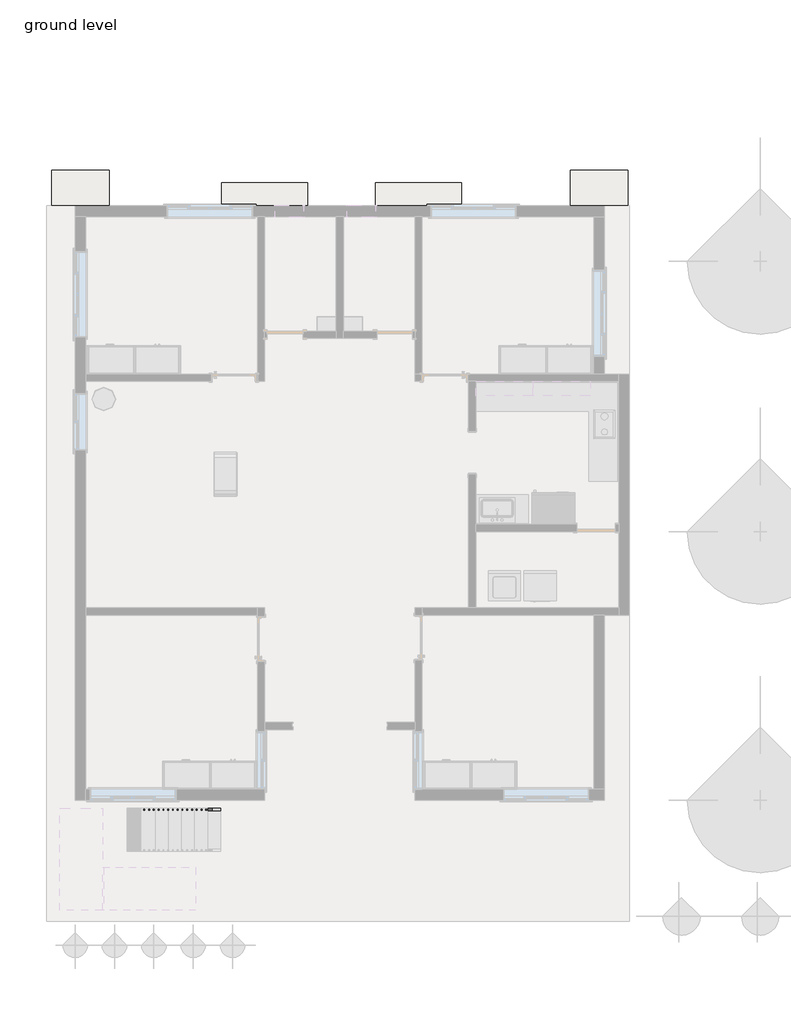
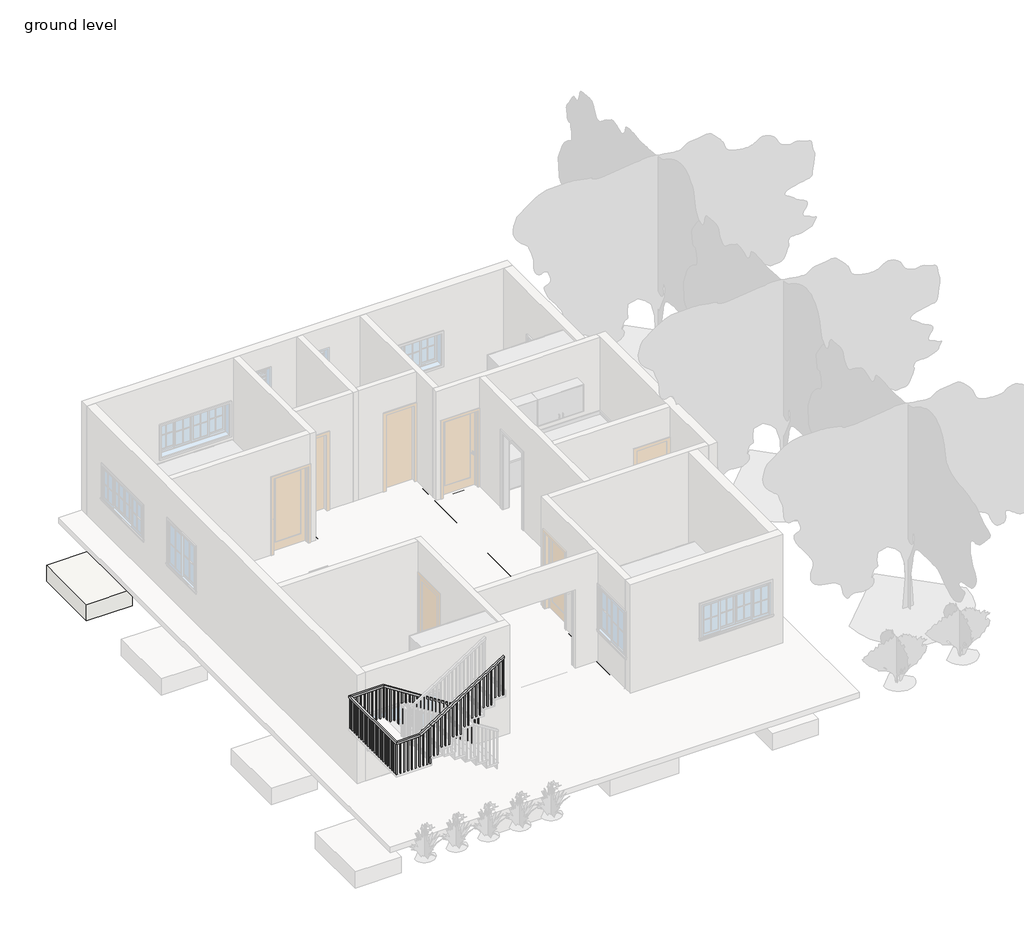
# One storey, part 2 of 4: 7 slabs, 6 beams, 1 railing.
"""IFC4 building model written with IfcOpenShell, lengths in millimetres."""

from ifc_helpers import new_model, si_unit, frame, origin, place, context, project, spatial, polyline, outline, extrude, faceted_brep, element, save

model = new_model("IFC4")

# Units and contexts
model_context = context("Model", 3, world=origin())
ifc_project = project(units=[si_unit("LENGTHUNIT", "METRE", prefix="MILLI")], contexts=[model_context])

# Site, building, storey
site = spatial("IfcSite", under=ifc_project)
building = spatial("IfcBuilding", under=site)
storey = spatial("IfcBuildingStorey", under=building, Name="ground level", Elevation=609.6)

# Beams
placement = place(None, origin())
element("IfcBeam", 1, ObjectType="Concrete-Rectangular Beam", at=placement, inside=storey, context=model_context, shape_type="Brep", body=[
    faceted_brep([(-12413.6124084, 10142.6961804, 609.6), (-12413.6124084, 9914.0961804, 609.6), (-8794.1124084, 9914.0961804, 609.6), (-8565.5124084, 9914.0961804, 609.6), (-7117.7124084, 9914.0961804, 609.6), (-6889.1124084, 9914.0961804, 609.6), (-5441.3124084, 9914.0961804, 609.6), (-5212.7124084, 9914.0961804, 609.6), (-1593.2124084, 9914.0961804, 609.6), (-1593.2124084, 10142.6961804, 609.6), (-5174.6124084, 10142.6961804, 609.6), (-5174.6124084, 9952.1961804, 609.6), (-5479.4124084, 9952.1961804, 609.6), (-5479.4124084, 10142.6961804, 609.6), (-8451.2124084, 10142.6961804, 609.6), (-8451.2124084, 9952.1961804, 609.6), (-8756.0124084, 9952.1961804, 609.6), (-8756.0124084, 10142.6961804, 609.6), (-12413.6124084, 9914.0961804, 304.8), (-8794.1124084, 9914.0961804, 304.8), (-8565.5124084, 9914.0961804, 304.8), (-7117.7124084, 9914.0961804, 304.8), (-6889.1124084, 9914.0961804, 304.8), (-5441.3124084, 9914.0961804, 304.8), (-5212.7124084, 9914.0961804, 304.8), (-1593.2124084, 9914.0961804, 304.8), (-12413.6124084, 10142.6961804, 304.8), (-8756.0124084, 10142.6961804, 304.8), (-8756.0124084, 9952.1961804, 304.8), (-8451.2124084, 9952.1961804, 304.8), (-8451.2124084, 10142.6961804, 304.8), (-5479.4124084, 10142.6961804, 304.8), (-5479.4124084, 9952.1961804, 304.8), (-5174.6124084, 9952.1961804, 304.8), (-5174.6124084, 10142.6961804, 304.8), (-1593.2124084, 10142.6961804, 304.8)], [[[0, 1, 2, 3, 4, 5, 6, 7, 8, 9, 10, 11, 12, 13, 14, 15, 16, 17]], [[1, 18, 19, 20, 21, 22, 23, 24, 25, 8, 7, 6, 5, 4, 3, 2]], [[18, 26, 27, 28, 29, 30, 31, 32, 33, 34, 35, 25, 24, 23, 22, 21, 20, 19]], [[26, 0, 17, 27]], [[1, 0, 26, 18]], [[29, 15, 14, 30]], [[15, 29, 28, 16]], [[16, 28, 27, 17]], [[33, 11, 10, 34]], [[11, 33, 32, 12]], [[12, 32, 31, 13]], [[9, 8, 25, 35]], [[34, 10, 9, 35]], [[30, 14, 13, 31]]]),
])
element("IfcBeam", 2, ObjectType="Concrete-Rectangular Beam", at=placement, inside=storey, context=model_context, shape_type="SweptSolid", body=[
    extrude(outline(polyline([(-1593.2124084, 9875.9961804), (-1364.6124084, 9875.9961804), (-1364.6124084, 6751.7961804), (-1593.2124084, 6751.7961804), (-1593.2124084, 9875.9961804)])), frame((0.0, 0.0, 304.8), z_axis=(0.0, 0.0, 1.0), x_axis=(1.0, 0.0, 0.0)), (0.0, 0.0, 1.0), 304.8),
])
element("IfcBeam", 3, ObjectType="Concrete-Rectangular Beam", at=placement, inside=storey, context=model_context, shape_type="Brep", body=[
    faceted_brep([(-843.9124084, 6713.6961804, 609.6), (-843.9124084, 6485.0961804, 609.6), (-843.9124084, 6485.0961804, 304.8), (-843.9124084, 6713.6961804, 304.8), (-1364.6124084, 6713.6961804, 609.6), (-1364.6124084, 6485.0961804, 609.6), (-1364.6124084, 6485.0961804, 304.8), (-1364.6124084, 6713.6961804, 304.8)], [[[0, 1, 2, 3]], [[1, 0, 4, 5]], [[2, 1, 5, 6]], [[3, 2, 6, 7]], [[0, 3, 7, 4]], [[5, 4, 7, 6]]]),
    faceted_brep([(-12413.6124084, 6485.0961804, 609.6), (-12413.6124084, 6713.6961804, 609.6), (-12413.6124084, 6713.6961804, 304.8), (-12413.6124084, 6485.0961804, 304.8), (-8756.0124084, 6713.6961804, 609.6), (-8756.0124084, 6485.0961804, 609.6), (-8756.0124084, 6485.0961804, 304.8), (-8756.0124084, 6713.6961804, 304.8), (-8794.1124084, 6485.0961804, 609.6), (-8794.1124084, 6713.6961804, 609.6), (-8794.1124084, 6485.0961804, 304.8), (-8794.1124084, 6713.6961804, 304.8)], [[[0, 1, 2, 3]], [[4, 5, 6, 7]], [[1, 0, 8, 5, 4, 9]], [[0, 3, 10, 6, 5, 8]], [[3, 2, 11, 7, 6, 10]], [[2, 1, 9, 4, 7, 11]]]),
    faceted_brep([(-1593.2124084, 6713.6961804, 609.6), (-1593.2124084, 6485.0961804, 609.6), (-1593.2124084, 6485.0961804, 304.8), (-1593.2124084, 6713.6961804, 304.8), (-5250.8124084, 6485.0961804, 609.6), (-5250.8124084, 6713.6961804, 609.6), (-5250.8124084, 6713.6961804, 304.8), (-5250.8124084, 6485.0961804, 304.8), (-5212.7124084, 6713.6961804, 609.6), (-5212.7124084, 6485.0961804, 609.6), (-5212.7124084, 6485.0961804, 304.8), (-5212.7124084, 6713.6961804, 304.8)], [[[0, 1, 2, 3]], [[4, 5, 6, 7]], [[1, 0, 8, 5, 4, 9]], [[2, 1, 9, 4, 7, 10]], [[3, 2, 10, 7, 6, 11]], [[0, 3, 11, 6, 5, 8]]]),
    faceted_brep([(-8527.4124084, 6485.0961804, 609.6), (-8527.4124084, 6713.6961804, 609.6), (-8527.4124084, 6713.6961804, 304.8), (-8527.4124084, 6485.0961804, 304.8), (-5479.4124084, 6713.6961804, 609.6), (-5479.4124084, 6485.0961804, 609.6), (-5479.4124084, 6485.0961804, 304.8), (-5479.4124084, 6713.6961804, 304.8)], [[[0, 1, 2, 3]], [[4, 5, 6, 7]], [[1, 0, 5, 4]], [[0, 3, 6, 5]], [[3, 2, 7, 6]], [[2, 1, 4, 7]]]),
])
element("IfcBeam", 4, ObjectType="Concrete-Rectangular Beam", at=placement, inside=storey, context=model_context, shape_type="Brep", body=[
    faceted_brep([(-5212.7124084, 9914.0961804, 609.6), (-5441.3124084, 9914.0961804, 609.6), (-5441.3124084, 7551.8961804, 609.6), (-5441.3124084, 7323.2961804, 609.6), (-5441.3124084, 6751.7961804, 609.6), (-5250.8124084, 6751.7961804, 609.6), (-5250.8124084, 6713.6961804, 609.6), (-5212.7124084, 6713.6961804, 609.6), (-5212.7124084, 9914.0961804, 304.8), (-5212.7124084, 6713.6961804, 304.8), (-5441.3124084, 9914.0961804, 304.8), (-5250.8124084, 6713.6961804, 304.8), (-5250.8124084, 6751.7961804, 304.8), (-5441.3124084, 6751.7961804, 304.8), (-5441.3124084, 7323.2961804, 304.8), (-5441.3124084, 7551.8961804, 304.8)], [[[0, 1, 2, 3, 4, 5, 6, 7]], [[8, 0, 7, 9]], [[10, 8, 9, 11, 12, 13, 14, 15]], [[1, 10, 15, 14, 13, 4, 3, 2]], [[1, 0, 8, 10]], [[5, 12, 11, 6]], [[12, 5, 4, 13]], [[7, 6, 11, 9]]]),
    faceted_brep([(-5212.7124084, -2201.7038196, 609.6), (-5441.3124084, -2201.7038196, 609.6), (-5441.3124084, -2201.7038196, 304.8), (-5212.7124084, -2201.7038196, 304.8), (-5441.3124084, 1430.4961804, 609.6), (-5212.7124084, 1430.4961804, 609.6), (-5212.7124084, 1430.4961804, 304.8), (-5441.3124084, 1430.4961804, 304.8), (-5441.3124084, -779.3038196, 609.6), (-5441.3124084, -1007.9038196, 609.6), (-5441.3124084, -1007.9038196, 304.8), (-5441.3124084, -779.3038196, 304.8)], [[[0, 1, 2, 3]], [[4, 5, 6, 7]], [[1, 0, 5, 4, 8, 9]], [[3, 2, 10, 11, 7, 6]], [[0, 3, 6, 5]], [[2, 1, 9, 8, 4, 7, 11, 10]]]),
    faceted_brep([(-5250.8124084, 6446.9961804, 609.6), (-5250.8124084, 6446.9961804, 304.8), (-5441.3124084, 6446.9961804, 304.8), (-5441.3124084, 6446.9961804, 609.6), (-5403.2124084, 1697.1961804, 609.6), (-5403.2124084, 1697.1961804, 304.8), (-5212.7124084, 1697.1961804, 304.8), (-5212.7124084, 1697.1961804, 609.6), (-5403.2124084, 1659.0961804, 609.6), (-5403.2124084, 1659.0961804, 304.8), (-5250.8124084, 6485.0961804, 609.6), (-5212.7124084, 6485.0961804, 609.6), (-5212.7124084, 6485.0961804, 304.8), (-5250.8124084, 6485.0961804, 304.8), (-5441.3124084, 1659.0961804, 609.6), (-5441.3124084, 1659.0961804, 304.8)], [[[0, 1, 2, 3]], [[4, 5, 6, 7]], [[5, 4, 8, 9]], [[10, 11, 12, 13]], [[11, 10, 0, 3, 14, 8, 4, 7]], [[12, 11, 7, 6]], [[13, 12, 6, 5, 9, 15, 2, 1]], [[9, 8, 14, 15]], [[3, 2, 15, 14]], [[1, 0, 10, 13]]]),
])
element("IfcBeam", 5, ObjectType="Concrete-Rectangular Beam", at=placement, inside=storey, context=model_context, shape_type="SweptSolid", body=[
    extrude(outline(polyline([(-7117.7124084, 9914.0961804), (-6889.1124084, 9914.0961804), (-6889.1124084, 7551.8961804), (-7117.7124084, 7551.8961804), (-7117.7124084, 9914.0961804)])), frame((0.0, 0.0, 304.8), z_axis=(0.0, 0.0, 1.0), x_axis=(1.0, 0.0, 0.0)), (0.0, 0.0, 1.0), 304.8),
])
element("IfcBeam", 6, ObjectType="Concrete-Rectangular Beam", at=placement, inside=storey, context=model_context, shape_type="Brep", body=[
    faceted_brep([(-5441.3124084, 7323.2961804, 609.6), (-5441.3124084, 7551.8961804, 609.6), (-6889.1124084, 7551.8961804, 609.6), (-7117.7124084, 7551.8961804, 609.6), (-8565.5124084, 7551.8961804, 609.6), (-8565.5124084, 7323.2961804, 609.6), (-5441.3124084, 7323.2961804, 304.8), (-8565.5124084, 7323.2961804, 304.8), (-5441.3124084, 7551.8961804, 304.8), (-8565.5124084, 7551.8961804, 304.8), (-7117.7124084, 7551.8961804, 304.8), (-6889.1124084, 7551.8961804, 304.8)], [[[0, 1, 2, 3, 4, 5]], [[6, 0, 5, 7]], [[8, 6, 7, 9, 10, 11]], [[1, 8, 11, 10, 9, 4, 3, 2]], [[1, 0, 6, 8]], [[5, 4, 9, 7]]]),
])

# Railing
element("IfcRailing", 7, ObjectType="Handrail - Rectangular", at=placement, inside=storey, context=model_context, shape_type="SolidModel", body=[
    faceted_brep([(-9543.8120641, -2698.7669819, 1701.8), (-9543.8120641, -2698.7669819, 1641.586276), (-9543.8120641, -2647.9669819, 1641.586276), (-9543.8120641, -2647.9669819, 1701.8), (-12058.4120641, -2698.7669819, 3302.0), (-12073.205059, -2698.7669819, 3251.2), (-12073.205059, -2647.9669819, 3251.2), (-12058.4120641, -2647.9669819, 3302.0), (-12922.0120641, -2698.7669819, 3302.0), (-12922.0120641, -2698.7669819, 3251.2), (-12972.8120641, -2647.9669819, 3251.2), (-12972.8120641, -2647.9669819, 3302.0), (-12922.0120641, -4767.1038196, 3302.0), (-12922.0120641, -4767.1038196, 3251.2), (-12972.8120641, -4817.9038196, 3251.2), (-12972.8120641, -4817.9038196, 3302.0), (-12337.8120641, -4767.1038196, 3302.0), (-12323.0190691, -4767.1038196, 3251.2), (-12323.0190691, -4817.9038196, 3251.2), (-12337.8120641, -4817.9038196, 3302.0), (-12058.4120641, -4767.1038196, 3479.8), (-12031.138789, -4767.1038196, 3436.9419964), (-12031.138789, -4817.9038196, 3436.9419964), (-12058.4120641, -4817.9038196, 3479.8), (-10102.6120641, -4767.1038196, 4724.4), (-10102.6120641, -4817.9038196, 4724.4), (-10102.6120641, -4817.9038196, 4664.186276), (-10102.6120641, -4767.1038196, 4664.186276)], [[[0, 1, 2, 3]], [[1, 0, 4, 5]], [[2, 1, 5, 6]], [[3, 2, 6, 7]], [[0, 3, 7, 4]], [[5, 4, 8, 9]], [[6, 5, 9, 10]], [[7, 6, 10, 11]], [[4, 7, 11, 8]], [[9, 8, 12, 13]], [[10, 9, 13, 14]], [[11, 10, 14, 15]], [[8, 11, 15, 12]], [[13, 12, 16, 17]], [[14, 13, 17, 18]], [[15, 14, 18, 19]], [[12, 15, 19, 16]], [[17, 16, 20, 21]], [[18, 17, 21, 22]], [[19, 18, 22, 23]], [[16, 19, 23, 20]], [[24, 25, 26, 27]], [[21, 20, 24, 27]], [[22, 21, 27, 26]], [[23, 22, 26, 25]], [[20, 23, 25, 24]]]),
    extrude(outline(polyline([(4654.0840032, -10118.4870641), (4641.961276, -10137.5370641), (3632.2, -10137.5370641), (3632.2, -10118.4870641), (4654.0840032, -10118.4870641)])), frame((0.0, -4802.0288196, 0.0), z_axis=(0.0, 1.0, 0.0), x_axis=(0.0, 0.0, 1.0)), (0.0, 0.0, 1.0), 19.05),
    extrude(outline(polyline([(4589.4294578, -10220.0870641), (4577.3067305, -10239.1370641), (3632.2, -10239.1370641), (3632.2, -10220.0870641), (4589.4294578, -10220.0870641)])), frame((0.0, -4802.0288196, 0.0), z_axis=(0.0, 1.0, 0.0), x_axis=(0.0, 0.0, 1.0)), (0.0, 0.0, 1.0), 19.05),
    extrude(outline(polyline([(4524.7749123, -10321.6870641), (4512.6521851, -10340.7370641), (3632.2, -10340.7370641), (3632.2, -10321.6870641), (4524.7749123, -10321.6870641)])), frame((0.0, -4802.0288196, 0.0), z_axis=(0.0, 1.0, 0.0), x_axis=(0.0, 0.0, 1.0)), (0.0, 0.0, 1.0), 19.05),
    extrude(outline(polyline([(4460.1203669, -10423.2870641), (4447.9976396, -10442.3370641), (3454.4, -10442.3370641), (3454.4, -10423.2870641), (4460.1203669, -10423.2870641)])), frame((0.0, -4802.0288196, 0.0), z_axis=(0.0, 1.0, 0.0), x_axis=(0.0, 0.0, 1.0)), (0.0, 0.0, 1.0), 19.05),
    extrude(outline(polyline([(4395.4658214, -10524.8870641), (4383.3430941, -10543.9370641), (3454.4, -10543.9370641), (3454.4, -10524.8870641), (4395.4658214, -10524.8870641)])), frame((0.0, -4802.0288196, 0.0), z_axis=(0.0, 1.0, 0.0), x_axis=(0.0, 0.0, 1.0)), (0.0, 0.0, 1.0), 19.05),
    extrude(outline(polyline([(4330.811276, -10626.4870641), (4318.6885487, -10645.5370641), (3454.4, -10645.5370641), (3454.4, -10626.4870641), (4330.811276, -10626.4870641)])), frame((0.0, -4802.0288196, 0.0), z_axis=(0.0, 1.0, 0.0), x_axis=(0.0, 0.0, 1.0)), (0.0, 0.0, 1.0), 19.05),
    extrude(outline(polyline([(4266.1567305, -10728.0870641), (4254.0340032, -10747.1370641), (3276.6, -10747.1370641), (3276.6, -10728.0870641), (4266.1567305, -10728.0870641)])), frame((0.0, -4802.0288196, 0.0), z_axis=(0.0, 1.0, 0.0), x_axis=(0.0, 0.0, 1.0)), (0.0, 0.0, 1.0), 19.05),
    extrude(outline(polyline([(4201.5021851, -10829.6870641), (4189.3794578, -10848.7370641), (3276.6, -10848.7370641), (3276.6, -10829.6870641), (4201.5021851, -10829.6870641)])), frame((0.0, -4802.0288196, 0.0), z_axis=(0.0, 1.0, 0.0), x_axis=(0.0, 0.0, 1.0)), (0.0, 0.0, 1.0), 19.05),
    extrude(outline(polyline([(4136.8476396, -10931.2870641), (4124.7249123, -10950.3370641), (3276.6, -10950.3370641), (3276.6, -10931.2870641), (4136.8476396, -10931.2870641)])), frame((0.0, -4802.0288196, 0.0), z_axis=(0.0, 1.0, 0.0), x_axis=(0.0, 0.0, 1.0)), (0.0, 0.0, 1.0), 19.05),
    extrude(outline(polyline([(4072.1930941, -11032.8870641), (4060.0703669, -11051.9370641), (3098.8, -11051.9370641), (3098.8, -11032.8870641), (4072.1930941, -11032.8870641)])), frame((0.0, -4802.0288196, 0.0), z_axis=(0.0, 1.0, 0.0), x_axis=(0.0, 0.0, 1.0)), (0.0, 0.0, 1.0), 19.05),
    extrude(outline(polyline([(4007.5385487, -11134.4870641), (3995.4158214, -11153.5370641), (3098.8, -11153.5370641), (3098.8, -11134.4870641), (4007.5385487, -11134.4870641)])), frame((0.0, -4802.0288196, 0.0), z_axis=(0.0, 1.0, 0.0), x_axis=(0.0, 0.0, 1.0)), (0.0, 0.0, 1.0), 19.05),
    extrude(outline(polyline([(3942.8840032, -11236.0870641), (3930.761276, -11255.1370641), (2921.0, -11255.1370641), (2921.0, -11236.0870641), (3942.8840032, -11236.0870641)])), frame((0.0, -4802.0288196, 0.0), z_axis=(0.0, 1.0, 0.0), x_axis=(0.0, 0.0, 1.0)), (0.0, 0.0, 1.0), 19.05),
    extrude(outline(polyline([(3878.2294578, -11337.6870641), (3866.1067305, -11356.7370641), (2921.0, -11356.7370641), (2921.0, -11337.6870641), (3878.2294578, -11337.6870641)])), frame((0.0, -4802.0288196, 0.0), z_axis=(0.0, 1.0, 0.0), x_axis=(0.0, 0.0, 1.0)), (0.0, 0.0, 1.0), 19.05),
    extrude(outline(polyline([(3813.5749123, -11439.2870641), (3801.4521851, -11458.3370641), (2921.0, -11458.3370641), (2921.0, -11439.2870641), (3813.5749123, -11439.2870641)])), frame((0.0, -4802.0288196, 0.0), z_axis=(0.0, 1.0, 0.0), x_axis=(0.0, 0.0, 1.0)), (0.0, 0.0, 1.0), 19.05),
    extrude(outline(polyline([(3748.9203669, -11540.8870641), (3736.7976396, -11559.9370641), (2743.2, -11559.9370641), (2743.2, -11540.8870641), (3748.9203669, -11540.8870641)])), frame((0.0, -4802.0288196, 0.0), z_axis=(0.0, 1.0, 0.0), x_axis=(0.0, 0.0, 1.0)), (0.0, 0.0, 1.0), 19.05),
    extrude(outline(polyline([(3684.2658214, -11642.4870641), (3672.1430941, -11661.5370641), (2743.2, -11661.5370641), (2743.2, -11642.4870641), (3684.2658214, -11642.4870641)])), frame((0.0, -4802.0288196, 0.0), z_axis=(0.0, 1.0, 0.0), x_axis=(0.0, 0.0, 1.0)), (0.0, 0.0, 1.0), 19.05),
    extrude(outline(polyline([(3619.611276, -11744.0870641), (3607.4885487, -11763.1370641), (2743.2, -11763.1370641), (2743.2, -11744.0870641), (3619.611276, -11744.0870641)])), frame((0.0, -4802.0288196, 0.0), z_axis=(0.0, 1.0, 0.0), x_axis=(0.0, 0.0, 1.0)), (0.0, 0.0, 1.0), 19.05),
    extrude(outline(polyline([(3554.9567305, -11845.6870641), (3542.8340032, -11864.7370641), (2565.4, -11864.7370641), (2565.4, -11845.6870641), (3554.9567305, -11845.6870641)])), frame((0.0, -4802.0288196, 0.0), z_axis=(0.0, 1.0, 0.0), x_axis=(0.0, 0.0, 1.0)), (0.0, 0.0, 1.0), 19.05),
    extrude(outline(polyline([(3490.3021851, -11947.2870641), (3478.1794578, -11966.3370641), (2565.4, -11966.3370641), (2565.4, -11947.2870641), (3490.3021851, -11947.2870641)])), frame((0.0, -4802.0288196, 0.0), z_axis=(0.0, 1.0, 0.0), x_axis=(0.0, 0.0, 1.0)), (0.0, 0.0, 1.0), 19.05),
    extrude(outline(polyline([(3377.1567305, -12125.0870641), (3365.0340032, -12144.1370641), (2387.6, -12144.1370641), (2387.6, -12125.0870641), (3377.1567305, -12125.0870641)])), frame((0.0, -4802.0288196, 0.0), z_axis=(0.0, 1.0, 0.0), x_axis=(0.0, 0.0, 1.0)), (0.0, 0.0, 1.0), 19.05),
    extrude(outline(polyline([(3312.5021851, -12226.6870641), (3300.3794578, -12245.7370641), (2387.6, -12245.7370641), (2387.6, -12226.6870641), (3312.5021851, -12226.6870641)])), frame((0.0, -4802.0288196, 0.0), z_axis=(0.0, 1.0, 0.0), x_axis=(0.0, 0.0, 1.0)), (0.0, 0.0, 1.0), 19.05),
    extrude(outline(polyline([(-12347.3370641, -4802.0288196), (-12347.3370641, -4782.9788196), (-12328.2870641, -4782.9788196), (-12328.2870641, -4802.0288196), (-12347.3370641, -4802.0288196)])), frame((0.0, 0.0, 2387.6), z_axis=(0.0, 0.0, 1.0), x_axis=(1.0, 0.0, 0.0)), (0.0, 0.0, 1.0), 863.6),
    extrude(outline(polyline([(-12448.9370641, -4802.0288196), (-12448.9370641, -4782.9788196), (-12429.8870641, -4782.9788196), (-12429.8870641, -4802.0288196), (-12448.9370641, -4802.0288196)])), frame((0.0, 0.0, 2387.6), z_axis=(0.0, 0.0, 1.0), x_axis=(1.0, 0.0, 0.0)), (0.0, 0.0, 1.0), 863.6),
    extrude(outline(polyline([(-12550.5370641, -4802.0288196), (-12550.5370641, -4782.9788196), (-12531.4870641, -4782.9788196), (-12531.4870641, -4802.0288196), (-12550.5370641, -4802.0288196)])), frame((0.0, 0.0, 2387.6), z_axis=(0.0, 0.0, 1.0), x_axis=(1.0, 0.0, 0.0)), (0.0, 0.0, 1.0), 863.6),
    extrude(outline(polyline([(-12652.1370641, -4802.0288196), (-12652.1370641, -4782.9788196), (-12633.0870641, -4782.9788196), (-12633.0870641, -4802.0288196), (-12652.1370641, -4802.0288196)])), frame((0.0, 0.0, 2387.6), z_axis=(0.0, 0.0, 1.0), x_axis=(1.0, 0.0, 0.0)), (0.0, 0.0, 1.0), 863.6),
    extrude(outline(polyline([(-12753.7370641, -4802.0288196), (-12753.7370641, -4782.9788196), (-12734.6870641, -4782.9788196), (-12734.6870641, -4802.0288196), (-12753.7370641, -4802.0288196)])), frame((0.0, 0.0, 2387.6), z_axis=(0.0, 0.0, 1.0), x_axis=(1.0, 0.0, 0.0)), (0.0, 0.0, 1.0), 863.6),
    extrude(outline(polyline([(-12855.3370641, -4802.0288196), (-12855.3370641, -4782.9788196), (-12836.2870641, -4782.9788196), (-12836.2870641, -4802.0288196), (-12855.3370641, -4802.0288196)])), frame((0.0, 0.0, 2387.6), z_axis=(0.0, 0.0, 1.0), x_axis=(1.0, 0.0, 0.0)), (0.0, 0.0, 1.0), 863.6),
    extrude(outline(polyline([(-12956.9370641, -4695.8419819), (-12937.8870641, -4695.8419819), (-12937.8870641, -4714.8919819), (-12956.9370641, -4714.8919819), (-12956.9370641, -4695.8419819)])), frame((0.0, 0.0, 2387.6), z_axis=(0.0, 0.0, 1.0), x_axis=(1.0, 0.0, 0.0)), (0.0, 0.0, 1.0), 863.6),
    extrude(outline(polyline([(-12956.9370641, -4594.2419819), (-12937.8870641, -4594.2419819), (-12937.8870641, -4613.2919819), (-12956.9370641, -4613.2919819), (-12956.9370641, -4594.2419819)])), frame((0.0, 0.0, 2387.6), z_axis=(0.0, 0.0, 1.0), x_axis=(1.0, 0.0, 0.0)), (0.0, 0.0, 1.0), 863.6),
    extrude(outline(polyline([(-12956.9370641, -4492.6419819), (-12937.8870641, -4492.6419819), (-12937.8870641, -4511.6919819), (-12956.9370641, -4511.6919819), (-12956.9370641, -4492.6419819)])), frame((0.0, 0.0, 2387.6), z_axis=(0.0, 0.0, 1.0), x_axis=(1.0, 0.0, 0.0)), (0.0, 0.0, 1.0), 863.6),
    extrude(outline(polyline([(-12956.9370641, -4391.0419819), (-12937.8870641, -4391.0419819), (-12937.8870641, -4410.0919819), (-12956.9370641, -4410.0919819), (-12956.9370641, -4391.0419819)])), frame((0.0, 0.0, 2387.6), z_axis=(0.0, 0.0, 1.0), x_axis=(1.0, 0.0, 0.0)), (0.0, 0.0, 1.0), 863.6),
    extrude(outline(polyline([(-12956.9370641, -4289.4419819), (-12937.8870641, -4289.4419819), (-12937.8870641, -4308.4919819), (-12956.9370641, -4308.4919819), (-12956.9370641, -4289.4419819)])), frame((0.0, 0.0, 2387.6), z_axis=(0.0, 0.0, 1.0), x_axis=(1.0, 0.0, 0.0)), (0.0, 0.0, 1.0), 863.6),
    extrude(outline(polyline([(-12956.9370641, -4187.8419819), (-12937.8870641, -4187.8419819), (-12937.8870641, -4206.8919819), (-12956.9370641, -4206.8919819), (-12956.9370641, -4187.8419819)])), frame((0.0, 0.0, 2387.6), z_axis=(0.0, 0.0, 1.0), x_axis=(1.0, 0.0, 0.0)), (0.0, 0.0, 1.0), 863.6),
    extrude(outline(polyline([(-12956.9370641, -4086.2419819), (-12937.8870641, -4086.2419819), (-12937.8870641, -4105.2919819), (-12956.9370641, -4105.2919819), (-12956.9370641, -4086.2419819)])), frame((0.0, 0.0, 2387.6), z_axis=(0.0, 0.0, 1.0), x_axis=(1.0, 0.0, 0.0)), (0.0, 0.0, 1.0), 863.6),
    extrude(outline(polyline([(-12956.9370641, -3984.6419819), (-12937.8870641, -3984.6419819), (-12937.8870641, -4003.6919819), (-12956.9370641, -4003.6919819), (-12956.9370641, -3984.6419819)])), frame((0.0, 0.0, 2387.6), z_axis=(0.0, 0.0, 1.0), x_axis=(1.0, 0.0, 0.0)), (0.0, 0.0, 1.0), 863.6),
    extrude(outline(polyline([(-12956.9370641, -3883.0419819), (-12937.8870641, -3883.0419819), (-12937.8870641, -3902.0919819), (-12956.9370641, -3902.0919819), (-12956.9370641, -3883.0419819)])), frame((0.0, 0.0, 2387.6), z_axis=(0.0, 0.0, 1.0), x_axis=(1.0, 0.0, 0.0)), (0.0, 0.0, 1.0), 863.6),
    extrude(outline(polyline([(-12956.9370641, -3781.4419819), (-12937.8870641, -3781.4419819), (-12937.8870641, -3800.4919819), (-12956.9370641, -3800.4919819), (-12956.9370641, -3781.4419819)])), frame((0.0, 0.0, 2387.6), z_axis=(0.0, 0.0, 1.0), x_axis=(1.0, 0.0, 0.0)), (0.0, 0.0, 1.0), 863.6),
    extrude(outline(polyline([(-12956.9370641, -3679.8419819), (-12937.8870641, -3679.8419819), (-12937.8870641, -3698.8919819), (-12956.9370641, -3698.8919819), (-12956.9370641, -3679.8419819)])), frame((0.0, 0.0, 2387.6), z_axis=(0.0, 0.0, 1.0), x_axis=(1.0, 0.0, 0.0)), (0.0, 0.0, 1.0), 863.6),
    extrude(outline(polyline([(-12956.9370641, -3578.2419819), (-12937.8870641, -3578.2419819), (-12937.8870641, -3597.2919819), (-12956.9370641, -3597.2919819), (-12956.9370641, -3578.2419819)])), frame((0.0, 0.0, 2387.6), z_axis=(0.0, 0.0, 1.0), x_axis=(1.0, 0.0, 0.0)), (0.0, 0.0, 1.0), 863.6),
    extrude(outline(polyline([(-12956.9370641, -3476.6419819), (-12937.8870641, -3476.6419819), (-12937.8870641, -3495.6919819), (-12956.9370641, -3495.6919819), (-12956.9370641, -3476.6419819)])), frame((0.0, 0.0, 2387.6), z_axis=(0.0, 0.0, 1.0), x_axis=(1.0, 0.0, 0.0)), (0.0, 0.0, 1.0), 863.6),
    extrude(outline(polyline([(-12956.9370641, -3375.0419819), (-12937.8870641, -3375.0419819), (-12937.8870641, -3394.0919819), (-12956.9370641, -3394.0919819), (-12956.9370641, -3375.0419819)])), frame((0.0, 0.0, 2387.6), z_axis=(0.0, 0.0, 1.0), x_axis=(1.0, 0.0, 0.0)), (0.0, 0.0, 1.0), 863.6),
    extrude(outline(polyline([(-12956.9370641, -3273.4419819), (-12937.8870641, -3273.4419819), (-12937.8870641, -3292.4919819), (-12956.9370641, -3292.4919819), (-12956.9370641, -3273.4419819)])), frame((0.0, 0.0, 2387.6), z_axis=(0.0, 0.0, 1.0), x_axis=(1.0, 0.0, 0.0)), (0.0, 0.0, 1.0), 863.6),
    extrude(outline(polyline([(-12956.9370641, -3171.8419819), (-12937.8870641, -3171.8419819), (-12937.8870641, -3190.8919819), (-12956.9370641, -3190.8919819), (-12956.9370641, -3171.8419819)])), frame((0.0, 0.0, 2387.6), z_axis=(0.0, 0.0, 1.0), x_axis=(1.0, 0.0, 0.0)), (0.0, 0.0, 1.0), 863.6),
    extrude(outline(polyline([(-12956.9370641, -3070.2419819), (-12937.8870641, -3070.2419819), (-12937.8870641, -3089.2919819), (-12956.9370641, -3089.2919819), (-12956.9370641, -3070.2419819)])), frame((0.0, 0.0, 2387.6), z_axis=(0.0, 0.0, 1.0), x_axis=(1.0, 0.0, 0.0)), (0.0, 0.0, 1.0), 863.6),
    extrude(outline(polyline([(-12956.9370641, -2968.6419819), (-12937.8870641, -2968.6419819), (-12937.8870641, -2987.6919819), (-12956.9370641, -2987.6919819), (-12956.9370641, -2968.6419819)])), frame((0.0, 0.0, 2387.6), z_axis=(0.0, 0.0, 1.0), x_axis=(1.0, 0.0, 0.0)), (0.0, 0.0, 1.0), 863.6),
    extrude(outline(polyline([(-12956.9370641, -2867.0419819), (-12937.8870641, -2867.0419819), (-12937.8870641, -2886.0919819), (-12956.9370641, -2886.0919819), (-12956.9370641, -2867.0419819)])), frame((0.0, 0.0, 2387.6), z_axis=(0.0, 0.0, 1.0), x_axis=(1.0, 0.0, 0.0)), (0.0, 0.0, 1.0), 863.6),
    extrude(outline(polyline([(-12956.9370641, -2765.4419819), (-12937.8870641, -2765.4419819), (-12937.8870641, -2784.4919819), (-12956.9370641, -2784.4919819), (-12956.9370641, -2765.4419819)])), frame((0.0, 0.0, 2387.6), z_axis=(0.0, 0.0, 1.0), x_axis=(1.0, 0.0, 0.0)), (0.0, 0.0, 1.0), 863.6),
    extrude(outline(polyline([(-12861.6870641, -2663.8419819), (-12861.6870641, -2682.8919819), (-12880.7370641, -2682.8919819), (-12880.7370641, -2663.8419819), (-12861.6870641, -2663.8419819)])), frame((0.0, 0.0, 2387.6), z_axis=(0.0, 0.0, 1.0), x_axis=(1.0, 0.0, 0.0)), (0.0, 0.0, 1.0), 863.6),
    extrude(outline(polyline([(-12760.0870641, -2663.8419819), (-12760.0870641, -2682.8919819), (-12779.1370641, -2682.8919819), (-12779.1370641, -2663.8419819), (-12760.0870641, -2663.8419819)])), frame((0.0, 0.0, 2387.6), z_axis=(0.0, 0.0, 1.0), x_axis=(1.0, 0.0, 0.0)), (0.0, 0.0, 1.0), 863.6),
    extrude(outline(polyline([(-12658.4870641, -2663.8419819), (-12658.4870641, -2682.8919819), (-12677.5370641, -2682.8919819), (-12677.5370641, -2663.8419819), (-12658.4870641, -2663.8419819)])), frame((0.0, 0.0, 2387.6), z_axis=(0.0, 0.0, 1.0), x_axis=(1.0, 0.0, 0.0)), (0.0, 0.0, 1.0), 863.6),
    extrude(outline(polyline([(-12556.8870641, -2663.8419819), (-12556.8870641, -2682.8919819), (-12575.9370641, -2682.8919819), (-12575.9370641, -2663.8419819), (-12556.8870641, -2663.8419819)])), frame((0.0, 0.0, 2387.6), z_axis=(0.0, 0.0, 1.0), x_axis=(1.0, 0.0, 0.0)), (0.0, 0.0, 1.0), 863.6),
    extrude(outline(polyline([(-12455.2870641, -2663.8419819), (-12455.2870641, -2682.8919819), (-12474.3370641, -2682.8919819), (-12474.3370641, -2663.8419819), (-12455.2870641, -2663.8419819)])), frame((0.0, 0.0, 2387.6), z_axis=(0.0, 0.0, 1.0), x_axis=(1.0, 0.0, 0.0)), (0.0, 0.0, 1.0), 863.6),
    extrude(outline(polyline([(-12353.6870641, -2663.8419819), (-12353.6870641, -2682.8919819), (-12372.7370641, -2682.8919819), (-12372.7370641, -2663.8419819), (-12353.6870641, -2663.8419819)])), frame((0.0, 0.0, 2387.6), z_axis=(0.0, 0.0, 1.0), x_axis=(1.0, 0.0, 0.0)), (0.0, 0.0, 1.0), 863.6),
    extrude(outline(polyline([(-12252.0870641, -2663.8419819), (-12252.0870641, -2682.8919819), (-12271.1370641, -2682.8919819), (-12271.1370641, -2663.8419819), (-12252.0870641, -2663.8419819)])), frame((0.0, 0.0, 2387.6), z_axis=(0.0, 0.0, 1.0), x_axis=(1.0, 0.0, 0.0)), (0.0, 0.0, 1.0), 863.6),
    extrude(outline(polyline([(-12150.4870641, -2663.8419819), (-12150.4870641, -2682.8919819), (-12169.5370641, -2682.8919819), (-12169.5370641, -2663.8419819), (-12150.4870641, -2663.8419819)])), frame((0.0, 0.0, 2387.6), z_axis=(0.0, 0.0, 1.0), x_axis=(1.0, 0.0, 0.0)), (0.0, 0.0, 1.0), 863.6),
    extrude(outline(polyline([(3187.2340032, -11972.6870641), (3199.3567305, -11991.7370641), (2209.8, -11991.7370641), (2209.8, -11972.6870641), (3187.2340032, -11972.6870641)])), frame((0.0, -2682.8919819, 0.0), z_axis=(0.0, 1.0, 0.0), x_axis=(0.0, 0.0, 1.0)), (0.0, 0.0, 1.0), 19.05),
    extrude(outline(polyline([(3122.5794578, -11871.0870641), (3134.7021851, -11890.1370641), (2209.8, -11890.1370641), (2209.8, -11871.0870641), (3122.5794578, -11871.0870641)])), frame((0.0, -2682.8919819, 0.0), z_axis=(0.0, 1.0, 0.0), x_axis=(0.0, 0.0, 1.0)), (0.0, 0.0, 1.0), 19.05),
    extrude(outline(polyline([(3057.9249123, -11769.4870641), (3070.0476396, -11788.5370641), (2209.8, -11788.5370641), (2209.8, -11769.4870641), (3057.9249123, -11769.4870641)])), frame((0.0, -2682.8919819, 0.0), z_axis=(0.0, 1.0, 0.0), x_axis=(0.0, 0.0, 1.0)), (0.0, 0.0, 1.0), 19.05),
    extrude(outline(polyline([(2993.2703669, -11667.8870641), (3005.3930941, -11686.9370641), (2032.0, -11686.9370641), (2032.0, -11667.8870641), (2993.2703669, -11667.8870641)])), frame((0.0, -2682.8919819, 0.0), z_axis=(0.0, 1.0, 0.0), x_axis=(0.0, 0.0, 1.0)), (0.0, 0.0, 1.0), 19.05),
    extrude(outline(polyline([(2928.6158214, -11566.2870641), (2940.7385487, -11585.3370641), (2032.0, -11585.3370641), (2032.0, -11566.2870641), (2928.6158214, -11566.2870641)])), frame((0.0, -2682.8919819, 0.0), z_axis=(0.0, 1.0, 0.0), x_axis=(0.0, 0.0, 1.0)), (0.0, 0.0, 1.0), 19.05),
    extrude(outline(polyline([(2863.961276, -11464.6870641), (2876.0840032, -11483.7370641), (1854.2, -11483.7370641), (1854.2, -11464.6870641), (2863.961276, -11464.6870641)])), frame((0.0, -2682.8919819, 0.0), z_axis=(0.0, 1.0, 0.0), x_axis=(0.0, 0.0, 1.0)), (0.0, 0.0, 1.0), 19.05),
    extrude(outline(polyline([(2799.3067305, -11363.0870641), (2811.4294578, -11382.1370641), (1854.2, -11382.1370641), (1854.2, -11363.0870641), (2799.3067305, -11363.0870641)])), frame((0.0, -2682.8919819, 0.0), z_axis=(0.0, 1.0, 0.0), x_axis=(0.0, 0.0, 1.0)), (0.0, 0.0, 1.0), 19.05),
    extrude(outline(polyline([(2734.6521851, -11261.4870641), (2746.7749123, -11280.5370641), (1854.2, -11280.5370641), (1854.2, -11261.4870641), (2734.6521851, -11261.4870641)])), frame((0.0, -2682.8919819, 0.0), z_axis=(0.0, 1.0, 0.0), x_axis=(0.0, 0.0, 1.0)), (0.0, 0.0, 1.0), 19.05),
    extrude(outline(polyline([(2669.9976396, -11159.8870641), (2682.1203669, -11178.9370641), (1676.4, -11178.9370641), (1676.4, -11159.8870641), (2669.9976396, -11159.8870641)])), frame((0.0, -2682.8919819, 0.0), z_axis=(0.0, 1.0, 0.0), x_axis=(0.0, 0.0, 1.0)), (0.0, 0.0, 1.0), 19.05),
    extrude(outline(polyline([(2605.3430941, -11058.2870641), (2617.4658214, -11077.3370641), (1676.4, -11077.3370641), (1676.4, -11058.2870641), (2605.3430941, -11058.2870641)])), frame((0.0, -2682.8919819, 0.0), z_axis=(0.0, 1.0, 0.0), x_axis=(0.0, 0.0, 1.0)), (0.0, 0.0, 1.0), 19.05),
    extrude(outline(polyline([(2540.6885487, -10956.6870641), (2552.811276, -10975.7370641), (1676.4, -10975.7370641), (1676.4, -10956.6870641), (2540.6885487, -10956.6870641)])), frame((0.0, -2682.8919819, 0.0), z_axis=(0.0, 1.0, 0.0), x_axis=(0.0, 0.0, 1.0)), (0.0, 0.0, 1.0), 19.05),
    extrude(outline(polyline([(2476.0340032, -10855.0870641), (2488.1567305, -10874.1370641), (1498.6, -10874.1370641), (1498.6, -10855.0870641), (2476.0340032, -10855.0870641)])), frame((0.0, -2682.8919819, 0.0), z_axis=(0.0, 1.0, 0.0), x_axis=(0.0, 0.0, 1.0)), (0.0, 0.0, 1.0), 19.05),
    extrude(outline(polyline([(2411.3794578, -10753.4870641), (2423.5021851, -10772.5370641), (1498.6, -10772.5370641), (1498.6, -10753.4870641), (2411.3794578, -10753.4870641)])), frame((0.0, -2682.8919819, 0.0), z_axis=(0.0, 1.0, 0.0), x_axis=(0.0, 0.0, 1.0)), (0.0, 0.0, 1.0), 19.05),
    extrude(outline(polyline([(2346.7249123, -10651.8870641), (2358.8476396, -10670.9370641), (1498.6, -10670.9370641), (1498.6, -10651.8870641), (2346.7249123, -10651.8870641)])), frame((0.0, -2682.8919819, 0.0), z_axis=(0.0, 1.0, 0.0), x_axis=(0.0, 0.0, 1.0)), (0.0, 0.0, 1.0), 19.05),
    extrude(outline(polyline([(2282.0703669, -10550.2870641), (2294.1930941, -10569.3370641), (1320.8, -10569.3370641), (1320.8, -10550.2870641), (2282.0703669, -10550.2870641)])), frame((0.0, -2682.8919819, 0.0), z_axis=(0.0, 1.0, 0.0), x_axis=(0.0, 0.0, 1.0)), (0.0, 0.0, 1.0), 19.05),
    extrude(outline(polyline([(2217.4158214, -10448.6870641), (2229.5385487, -10467.7370641), (1320.8, -10467.7370641), (1320.8, -10448.6870641), (2217.4158214, -10448.6870641)])), frame((0.0, -2682.8919819, 0.0), z_axis=(0.0, 1.0, 0.0), x_axis=(0.0, 0.0, 1.0)), (0.0, 0.0, 1.0), 19.05),
    extrude(outline(polyline([(2152.761276, -10347.0870641), (2164.8840032, -10366.1370641), (1143.0, -10366.1370641), (1143.0, -10347.0870641), (2152.761276, -10347.0870641)])), frame((0.0, -2682.8919819, 0.0), z_axis=(0.0, 1.0, 0.0), x_axis=(0.0, 0.0, 1.0)), (0.0, 0.0, 1.0), 19.05),
    extrude(outline(polyline([(2088.1067305, -10245.4870641), (2100.2294578, -10264.5370641), (1143.0, -10264.5370641), (1143.0, -10245.4870641), (2088.1067305, -10245.4870641)])), frame((0.0, -2682.8919819, 0.0), z_axis=(0.0, 1.0, 0.0), x_axis=(0.0, 0.0, 1.0)), (0.0, 0.0, 1.0), 19.05),
    extrude(outline(polyline([(2023.4521851, -10143.8870641), (2035.5749123, -10162.9370641), (1143.0, -10162.9370641), (1143.0, -10143.8870641), (2023.4521851, -10143.8870641)])), frame((0.0, -2682.8919819, 0.0), z_axis=(0.0, 1.0, 0.0), x_axis=(0.0, 0.0, 1.0)), (0.0, 0.0, 1.0), 19.05),
    extrude(outline(polyline([(1958.7976396, -10042.2870641), (1970.9203669, -10061.3370641), (965.2, -10061.3370641), (965.2, -10042.2870641), (1958.7976396, -10042.2870641)])), frame((0.0, -2682.8919819, 0.0), z_axis=(0.0, 1.0, 0.0), x_axis=(0.0, 0.0, 1.0)), (0.0, 0.0, 1.0), 19.05),
    extrude(outline(polyline([(1894.1430941, -9940.6870641), (1906.2658214, -9959.7370641), (965.2, -9959.7370641), (965.2, -9940.6870641), (1894.1430941, -9940.6870641)])), frame((0.0, -2682.8919819, 0.0), z_axis=(0.0, 1.0, 0.0), x_axis=(0.0, 0.0, 1.0)), (0.0, 0.0, 1.0), 19.05),
    extrude(outline(polyline([(1829.4885487, -9839.0870641), (1841.611276, -9858.1370641), (965.2, -9858.1370641), (965.2, -9839.0870641), (1829.4885487, -9839.0870641)])), frame((0.0, -2682.8919819, 0.0), z_axis=(0.0, 1.0, 0.0), x_axis=(0.0, 0.0, 1.0)), (0.0, 0.0, 1.0), 19.05),
    extrude(outline(polyline([(1764.8340032, -9737.4870641), (1776.9567305, -9756.5370641), (787.4, -9756.5370641), (787.4, -9737.4870641), (1764.8340032, -9737.4870641)])), frame((0.0, -2682.8919819, 0.0), z_axis=(0.0, 1.0, 0.0), x_axis=(0.0, 0.0, 1.0)), (0.0, 0.0, 1.0), 19.05),
    extrude(outline(polyline([(1700.1794578, -9635.8870641), (1712.3021851, -9654.9370641), (787.4, -9654.9370641), (787.4, -9635.8870641), (1700.1794578, -9635.8870641)])), frame((0.0, -2682.8919819, 0.0), z_axis=(0.0, 1.0, 0.0), x_axis=(0.0, 0.0, 1.0)), (0.0, 0.0, 1.0), 19.05),
    extrude(outline(polyline([(3425.6476396, -12048.8870641), (3413.5249123, -12067.9370641), (2387.6, -12067.9370641), (2387.6, -12048.8870641), (3425.6476396, -12048.8870641)])), frame((0.0, -4802.0288196, 0.0), z_axis=(0.0, 1.0, 0.0), x_axis=(0.0, 0.0, 1.0)), (0.0, 0.0, 1.0), 19.05),
    extrude(outline(polyline([(-12956.9370641, -4782.9788196), (-12937.8870641, -4782.9788196), (-12937.8870641, -4802.0288196), (-12956.9370641, -4802.0288196), (-12956.9370641, -4782.9788196)])), frame((0.0, 0.0, 2387.6), z_axis=(0.0, 0.0, 1.0), x_axis=(1.0, 0.0, 0.0)), (0.0, 0.0, 1.0), 863.6),
    extrude(outline(polyline([(-12937.8870641, -2663.8419819), (-12937.8870641, -2682.8919819), (-12956.9370641, -2682.8919819), (-12956.9370641, -2663.8419819), (-12937.8870641, -2663.8419819)])), frame((0.0, 0.0, 2387.6), z_axis=(0.0, 0.0, 1.0), x_axis=(1.0, 0.0, 0.0)), (0.0, 0.0, 1.0), 863.6),
    extrude(outline(polyline([(3235.7249123, -12048.8870641), (3247.8476396, -12067.9370641), (2387.6, -12067.9370641), (2387.6, -12048.8870641), (3235.7249123, -12048.8870641)])), frame((0.0, -2682.8919819, 0.0), z_axis=(0.0, 1.0, 0.0), x_axis=(0.0, 0.0, 1.0)), (0.0, 0.0, 1.0), 19.05),
    extrude(outline(polyline([(4664.186276, -10102.6120641), (4652.0635487, -10121.6620641), (3632.2, -10121.6620641), (3632.2, -10102.6120641), (4664.186276, -10102.6120641)])), frame((0.0, -4802.0288196, 0.0), z_axis=(0.0, 1.0, 0.0), x_axis=(0.0, 0.0, 1.0)), (0.0, 0.0, 1.0), 19.05),
    extrude(outline(polyline([(1641.586276, -9543.8120641), (1653.7090032, -9562.8620641), (787.4, -9562.8620641), (787.4, -9543.8120641), (1641.586276, -9543.8120641)])), frame((0.0, -2682.8919819, 0.0), z_axis=(0.0, 1.0, 0.0), x_axis=(0.0, 0.0, 1.0)), (0.0, 0.0, 1.0), 19.05),
])

# Slabs
element("IfcSlab", 8, ObjectType="Footing-Rectangular : 72\" x 48\" x 18\"", at=placement, inside=storey, context=model_context, shape_type="SweptSolid", body=[
    extrude(outline(polyline([(-11918.3124084, 10942.7961804), (-11918.3124084, 9113.9961804), (-13137.5124084, 9113.9961804), (-13137.5124084, 10942.7961804), (-11918.3124084, 10942.7961804)])), frame((0.0, 0.0, -1676.4), z_axis=(0.0, 0.0, 1.0), x_axis=(1.0, 0.0, 0.0)), (0.0, 0.0, 1.0), 457.2),
])
element("IfcSlab", 9, ObjectType="Footing-Rectangular : 72\" x 48\" x 18\"", at=placement, inside=storey, context=model_context, shape_type="SweptSolid", body=[
    extrude(outline(polyline([(-9518.0124084, 10676.0961804), (-7689.2124084, 10676.0961804), (-7689.2124084, 9456.8961804), (-9518.0124084, 9456.8961804), (-9518.0124084, 10676.0961804)])), frame((0.0, 0.0, -1676.4), z_axis=(0.0, 0.0, 1.0), x_axis=(1.0, 0.0, 0.0)), (0.0, 0.0, 1.0), 457.2),
])
element("IfcSlab", 10, ObjectType="Footing-Rectangular : 72\" x 48\" x 18\"", at=placement, inside=storey, context=model_context, shape_type="SweptSolid", body=[
    extrude(outline(polyline([(-6241.4124084, 10676.0961804), (-4412.6124084, 10676.0961804), (-4412.6124084, 9456.8961804), (-6241.4124084, 9456.8961804), (-6241.4124084, 10676.0961804)])), frame((0.0, 0.0, -1676.4), z_axis=(0.0, 0.0, 1.0), x_axis=(1.0, 0.0, 0.0)), (0.0, 0.0, 1.0), 457.2),
])
element("IfcSlab", 11, ObjectType="Footing-Rectangular : 72\" x 48\" x 18\"", at=placement, inside=storey, context=model_context, shape_type="SweptSolid", body=[
    extrude(outline(polyline([(-869.3124084, 10942.7961804), (-869.3124084, 9113.9961804), (-2088.5124084, 9113.9961804), (-2088.5124084, 10942.7961804), (-869.3124084, 10942.7961804)])), frame((0.0, 0.0, -1676.4), z_axis=(0.0, 0.0, 1.0), x_axis=(1.0, 0.0, 0.0)), (0.0, 0.0, 1.0), 457.2),
])
element("IfcSlab", 12, ObjectType="Footing-Rectangular : 72\" x 48\" x 18\"", at=placement, inside=storey, context=model_context, shape_type="SweptSolid", body=[
    extrude(outline(polyline([(-869.3124084, 7513.7961804), (-869.3124084, 5684.9961804), (-2088.5124084, 5684.9961804), (-2088.5124084, 7513.7961804), (-869.3124084, 7513.7961804)])), frame((0.0, 0.0, -1676.4), z_axis=(0.0, 0.0, 1.0), x_axis=(1.0, 0.0, 0.0)), (0.0, 0.0, 1.0), 457.2),
])
element("IfcSlab", 13, ObjectType="Footing-Rectangular : 72\" x 48\" x 18\"", at=placement, inside=storey, context=model_context, shape_type="SweptSolid", body=[
    extrude(outline(polyline([(-869.3124084, 2382.9961804), (-869.3124084, 554.1961804), (-2088.5124084, 554.1961804), (-2088.5124084, 2382.9961804), (-869.3124084, 2382.9961804)])), frame((0.0, 0.0, -1676.4), z_axis=(0.0, 0.0, 1.0), x_axis=(1.0, 0.0, 0.0)), (0.0, 0.0, 1.0), 457.2),
])
element("IfcSlab", 14, ObjectType="Footing-Rectangular : 72\" x 48\" x 18\"", at=placement, inside=storey, context=model_context, shape_type="SweptSolid", body=[
    extrude(outline(polyline([(-4755.5124084, 7513.7961804), (-4755.5124084, 5684.9961804), (-5974.7124084, 5684.9961804), (-5974.7124084, 7513.7961804), (-4755.5124084, 7513.7961804)])), frame((0.0, 0.0, -1676.4), z_axis=(0.0, 0.0, 1.0), x_axis=(1.0, 0.0, 0.0)), (0.0, 0.0, 1.0), 457.2),
])

save(model, "model.ifc")

# Revit data of these elements
# Type "Concrete-Rectangular Beam"
#   Assembly Code = "B10"
#   Length [instance default] = 5' - 0"
#   b = 0' - 9"
#   h = 1' - 0"
#   Structural Material [instance default] = Concrete, Cast-in-Place gray
# Type "Handrail - Rectangular"
#   Assembly Code = "C2010400"
#   built-in parameter 1008612 = 0.0416667 (stored number, unit not read)
#   built-in parameter 1008611 = 0.0416667 (stored number, unit not read)
#   built-in parameter 1008609 = 0.333333 (stored number, unit not read)
#   built-in parameter 1008604 = 0.166667 (stored number, unit not read)
#   built-in parameter 1008603 = 0.166667 (stored number, unit not read)
#   Railing Height = 3' - 0"
#   built-in parameter 1008630 = 2
#   built-in parameter 1008610 = 2
#   built-in parameter 1008618 = Baluster - Square : 3/4"
# Type "Footing-Rectangular : 72\" x 48\" x 18\""
#   Assembly Code = "A1010100"
#   Width = 4' - 0"
#   Length = 6' - 0"
#   Foundation Thickness = 1' - 6"
#   Structural Material [instance default] = Concrete, Cast-in-Place gray
# Elements 1, 2, 3, 4, 5, 6 (IfcBeam, "Concrete-Rectangular Beam")
#   Structural Material = Concrete, Cast-in-Place gray
#   Phase Created = New Construction
#   Materials on its faces: "Concrete, Cast-in-Place gray"
# Element 7 (IfcRailing, "Handrail - Rectangular")
#   Phase Created = New Construction
# Elements 8, 9, 10, 11, 12, 13, 14 (IfcSlab, "Footing-Rectangular : 72\" x 48\" x 18\"")
#   Structural Material = Concrete, Cast-in-Place gray
#   Phase Created = New Construction
#   Materials on its faces: "Concrete, Cast-in-Place gray"
# Materials
#   "Concrete, Cast-in-Place gray": class "Concrete", colour RGB 192 192 192, transparency 0, Description = "Cast-in-place concrete", Cost = 0
